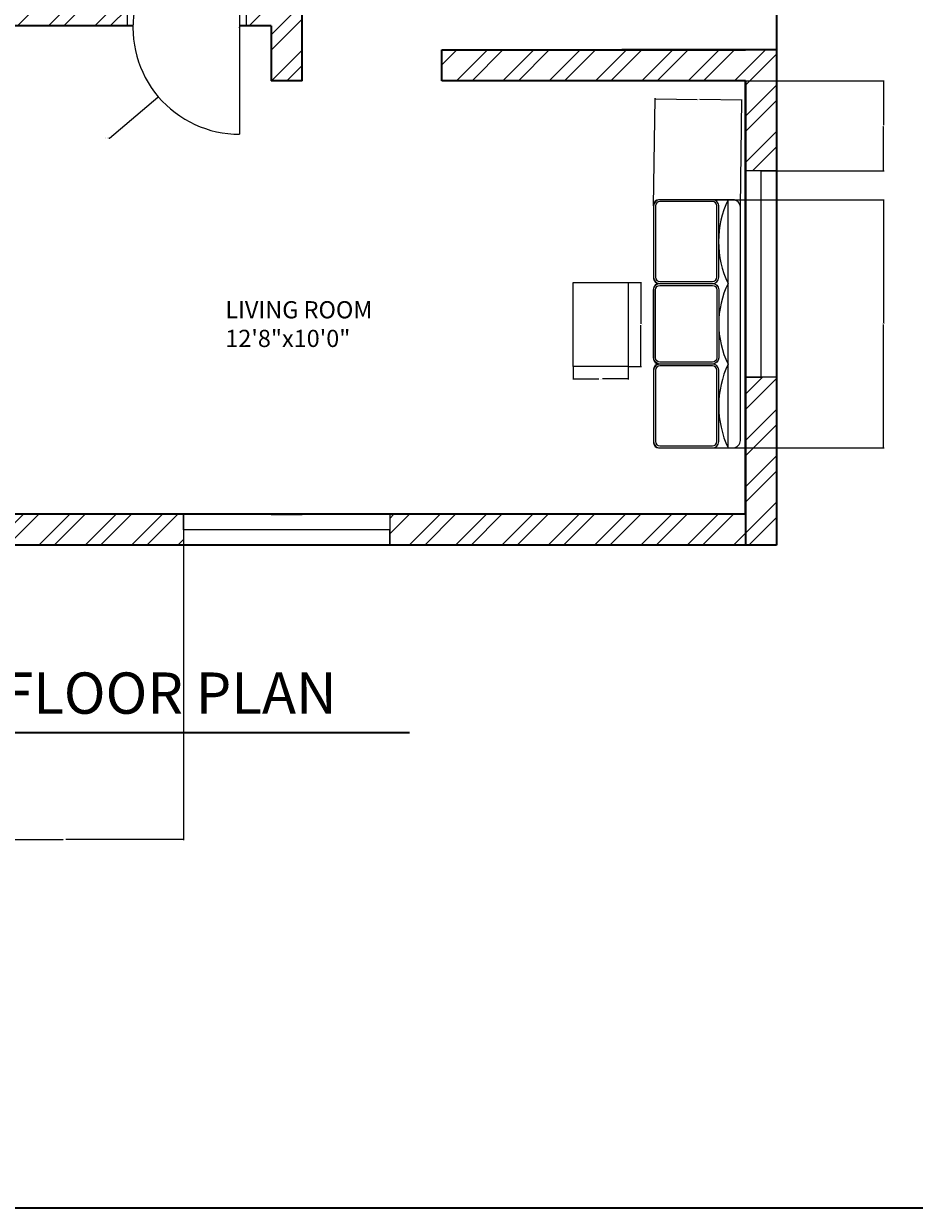
# Model space of a CAD drawing. Units: inches. Extents: x 1955 to 3324, y 980 to 3129.
# Tile 2 of 11: x 2296 to 2555, y 1704 to 2048. Entities that reach past the tile are written whole.
import ezdxf

# ---------------------------------------------------------------- set-up
doc = ezdxf.new("R2010")
doc.units = ezdxf.units.IN
for name, color, linetype, lineweight in [('A-ANNO-DIMS', 2, 'Continuous', 18), ('A-ANNO-TITL', 7, 'Continuous', 35), ('A-ANNO-TTLB', 7, 'Continuous', 35), ('A-AREA-IDEN', 7, 'Continuous', 18), ('A-DOOR', 3, 'Continuous', 18), ('A-FURN', 8, 'Continuous', 18), ('A-GLAZ', 4, 'Continuous', 18), ('A-WALL', 7, 'Continuous', 35), ('A-WALL-PATT', 252, 'Continuous', 13)]:
    doc.layers.add(name, color=color, linetype=linetype, lineweight=lineweight)
doc.styles.get("Standard").update_dxf_attribs({"font": 'arial.ttf'})
doc.dimstyles.get("Standard").update_dxf_attribs({"dimtxt": 0.18, "dimasz": 0.18, "dimexe": 0.18, "dimexo": 0.0625, "dimgap": 0.09, "dimtad": 0, "dimtih": 1, "dimtoh": 1, "dimdec": 4, "dimzin": 0, "dimdsep": 46, "dimtxsty": 'Standard', "dimcen": 0.09, "dimadec": 0, "dimazin": 0, "dimtfac": 1, "dimtdec": 4, "dimtofl": 0, "dimtmove": 0, "dimatfit": 3, "dimfxl": 1, "dimtolj": 1, "dimtzin": 0, "dimarcsym": 0})

# ---------------------------------------------------------------- blocks, each defined once
blk = doc.blocks.new('COFFEE-TABLE-RECT')
blk.add_lwpolyline([(0, 24.35), (16.02, 24.35), (16.02, 0), (0, 0)], close=True)
blk = doc.blocks.new('DOOR-UNIT-S')
for p, q in [((0, 31.5), (0, 40.5)), ((0, 40.5), (0, 36)), ((34.6, 31.5), (34.6, 40.5)), ((34.6, 40.5), (34.6, 36)), ((0, 36), (2, 36)), ((34.6, 36), (32.6, 36)), ((32.6, 36), (32.6, 0))]:
    blk.add_line(p, q)
blk.add_arc((32.6, 31.01), 31.01, 170.7301, 270)
blk = doc.blocks.new('WIN-PLAN-60-A')
for p, q in [((0, 60), (9, 60)), ((9, 60), (4.5, 60)), ((4.5, 60), (4.5, 0)), ((4.5, 0), (0, 0)), ((0, 0), (9, 0))]:
    blk.add_line(p, q)
blk = doc.blocks.new('*D57')
at = {"layer": 'A-ANNO-DIMS', "color": 0, "lineweight": -2, "transparency": 16777216}
for p, q in [((2472.15, 1972.84), (2475.92, 1972.84)), ((2475.74, 1972.66), (2475.74, 1960.85)), ((2475.74, 1948.67), (2475.74, 1960.49)), ((2472.15, 1948.49), (2475.92, 1948.49))]:
    blk.add_line(p, q, dxfattribs=at)
at = {"layer": 'A-ANNO-DIMS', "color": 0, "transparency": 16777216}
for points in [[(2475.71, 1972.66), (2475.77, 1972.66), (2475.74, 1972.84)], [(2475.71, 1948.67), (2475.77, 1948.67), (2475.74, 1948.49)]]:
    blk.add_solid(points, dxfattribs=at)
at = {"layer": 'Defpoints', "color": 0, "transparency": 16777216}
for p in [(2472.09, 1972.84), (2475.74, 1972.84), (2472.09, 1948.49)]:
    blk.add_point(p, dxfattribs=at)
at = {"layer": 'A-ANNO-DIMS', "color": 0, "transparency": 16777216, "insert": (2475.74, 1960.67), "char_height": 0.18, "attachment_point": 5}
blk.add_mtext('\\A1;TABLE 24 TYP.', dxfattribs=at)
blk = doc.blocks.new('*D58')
at = {"layer": 'A-ANNO-DIMS', "color": 0, "lineweight": -2, "transparency": 16777216}
for p, q in [((2456.07, 1948.43), (2456.07, 1944.66)), ((2472.09, 1948.43), (2472.09, 1944.66)), ((2456.25, 1944.84), (2463.56, 1944.84)), ((2471.91, 1944.84), (2464.6, 1944.84))]:
    blk.add_line(p, q, dxfattribs=at)
at = {"layer": 'A-ANNO-DIMS', "color": 0, "transparency": 16777216}
for points in [[(2456.25, 1944.87), (2456.25, 1944.81), (2456.07, 1944.84)], [(2471.91, 1944.87), (2471.91, 1944.81), (2472.09, 1944.84)]]:
    blk.add_solid(points, dxfattribs=at)
at = {"layer": 'Defpoints', "color": 0, "transparency": 16777216}
for p in [(2456.07, 1948.49), (2472.09, 1948.49), (2472.09, 1944.84)]:
    blk.add_point(p, dxfattribs=at)
at = {"layer": 'A-ANNO-DIMS', "color": 0, "transparency": 16777216, "insert": (2464.08, 1944.84), "char_height": 0.18, "attachment_point": 5}
blk.add_mtext('\\A1;16 TYP.', dxfattribs=at)
blk = doc.blocks.new('*D105')
at = {"layer": 'A-ANNO-DIMS', "color": 0, "lineweight": -2, "transparency": 16777216}
for p, q in [((2506.27, 2031.5), (2546.54, 2031.5)), ((2546.36, 2031.32), (2546.36, 2018.62)), ((2546.36, 2005.54), (2546.36, 2018.25)), ((2515.27, 2005.36), (2546.54, 2005.36))]:
    blk.add_line(p, q, dxfattribs=at)
at = {"layer": 'A-ANNO-DIMS', "color": 0, "transparency": 16777216}
for points in [[(2546.33, 2031.32), (2546.39, 2031.32), (2546.36, 2031.5)], [(2546.33, 2005.54), (2546.39, 2005.54), (2546.36, 2005.36)]]:
    blk.add_solid(points, dxfattribs=at)
at = {"layer": 'Defpoints', "color": 0, "transparency": 16777216}
for p in [(2506.21, 2031.5), (2546.36, 2031.5), (2515.21, 2005.36)]:
    blk.add_point(p, dxfattribs=at)
at = {"layer": 'A-ANNO-DIMS', "color": 0, "transparency": 16777216, "insert": (2546.36, 2018.43), "char_height": 0.18, "attachment_point": 5}
blk.add_mtext('\\A1;26.14', dxfattribs=at)
blk = doc.blocks.new('*D109')
at = {"layer": 'A-ANNO-DIMS', "color": 0, "lineweight": -2, "transparency": 16777216}
for p, q in [((2273.49, 1896.44), (2273.49, 1810.7)), ((2342.7, 1896.44), (2342.7, 1810.7)), ((2273.67, 1810.88), (2307.72, 1810.88)), ((2342.52, 1810.88), (2308.47, 1810.88))]:
    blk.add_line(p, q, dxfattribs=at)
at = {"layer": 'A-ANNO-DIMS', "color": 0, "transparency": 16777216}
for points in [[(2273.67, 1810.91), (2273.67, 1810.85), (2273.49, 1810.88)], [(2342.52, 1810.91), (2342.52, 1810.85), (2342.7, 1810.88)]]:
    blk.add_solid(points, dxfattribs=at)
at = {"layer": 'Defpoints', "color": 0, "transparency": 16777216}
for p in [(2273.49, 1896.5), (2342.7, 1896.5), (2342.7, 1810.88)]:
    blk.add_point(p, dxfattribs=at)
at = {"layer": 'A-ANNO-DIMS', "color": 0, "transparency": 16777216, "insert": (2308.09, 1810.88), "char_height": 0.18, "attachment_point": 5}
blk.add_mtext('\\A1;69.21', dxfattribs=at)
blk = doc.blocks.new('*D110')
at = {"layer": 'A-ANNO-DIMS', "color": 0, "lineweight": -2, "transparency": 16777216}
for p, q in [((2479.46, 1995.2), (2479.91, 2026.47)), ((2480.09, 2026.29), (2492.14, 2026.11)), ((2504.98, 2025.93), (2492.93, 2026.1)), ((2504.71, 1994.84), (2505.16, 2026.11))]:
    blk.add_line(p, q, dxfattribs=at)
at = {"layer": 'A-ANNO-DIMS', "color": 0, "transparency": 16777216}
for points in [[(2480.09, 2026.32), (2480.09, 2026.26), (2479.91, 2026.29)], [(2504.98, 2025.96), (2504.97, 2025.9), (2505.16, 2025.93)]]:
    blk.add_solid(points, dxfattribs=at)
at = {"layer": 'Defpoints', "color": 0, "transparency": 16777216}
for p in [(2505.16, 2025.93), (2479.46, 1995.14), (2504.71, 1994.78)]:
    blk.add_point(p, dxfattribs=at)
at = {"layer": 'A-ANNO-DIMS', "color": 0, "transparency": 16777216, "insert": (2492.53, 2026.11), "char_height": 0.18, "attachment_point": 5}
blk.add_mtext('\\A1;25.25', dxfattribs=at)
blk = doc.blocks.new('*D111')
at = {"layer": 'A-ANNO-DIMS', "color": 0, "lineweight": -2, "transparency": 16777216}
for p, q in [((2496.66, 1996.94), (2546.54, 1996.94)), ((2546.36, 1996.76), (2546.36, 1961.06)), ((2546.36, 1924.99), (2546.36, 1960.7)), ((2496.66, 1924.81), (2546.54, 1924.81))]:
    blk.add_line(p, q, dxfattribs=at)
at = {"layer": 'A-ANNO-DIMS', "color": 0, "transparency": 16777216}
for points in [[(2546.33, 1996.76), (2546.39, 1996.76), (2546.36, 1996.94)], [(2546.33, 1924.99), (2546.39, 1924.99), (2546.36, 1924.81)]]:
    blk.add_solid(points, dxfattribs=at)
at = {"layer": 'Defpoints', "color": 0, "transparency": 16777216}
for p in [(2496.6, 1996.94), (2546.36, 1996.94), (2496.6, 1924.81)]:
    blk.add_point(p, dxfattribs=at)
at = {"layer": 'A-ANNO-DIMS', "color": 0, "transparency": 16777216, "insert": (2546.36, 1960.88), "char_height": 0.18, "attachment_point": 5}
blk.add_mtext('\\A1;72.13', dxfattribs=at)
blk = doc.blocks.new('*D140')
at = {"layer": 'A-ANNO-DIMS', "color": 0, "lineweight": -2, "transparency": 16777216}
for p, q in [((2358.92, 2047), (2359.1, 2047)), ((2359.01, 2046.91), (2359.01, 2047.09)), ((2321.21, 2014.87), (2335.25, 2026.8)), ((2321.03, 2014.87), (2321.21, 2014.87))]:
    blk.add_line(p, q, dxfattribs=at)
at = {"layer": 'A-ANNO-DIMS', "color": 0, "transparency": 16777216}
blk.add_solid([(2335.23, 2026.82), (2335.27, 2026.78), (2335.39, 2026.92)], dxfattribs=at)
at = {"layer": 'Defpoints', "color": 0, "transparency": 16777216}
for p in [(2359.01, 2047), (2335.39, 2026.92)]:
    blk.add_point(p, dxfattribs=at)
at = {"layer": 'A-ANNO-DIMS', "color": 0, "transparency": 16777216, "insert": (2320.48, 2014.87), "char_height": 0.18, "attachment_point": 5}
blk.add_mtext('\\A1;R31.005', dxfattribs=at)

msp = doc.modelspace()

# ---------------------------------------------------------------- hatches: boundary and pattern name
at = {"layer": 'A-WALL-PATT'}
h = msp.add_hatch(dxfattribs=at)
h.set_pattern_fill('ANSI32', color=256)
h.paths.add_polyline_path([(2361.4775, 2456.5037), (2270.2755, 2456.5037), (2270.2755, 2447.5037), (2285.7102, 2447.5037), (2285.7102, 2363.5037), (2281.1795, 2363.5037), (2281.1795, 2359.0037), (2290.2102, 2359.0037), (2290.2102, 2447.5037), (2361.4775, 2447.5037), (2361.4775, 2452.0037)])
h.paths.add_polyline_path([(2246.2755, 2456.5037), (2197.6809, 2456.5037), (2197.6809, 2447.5037), (2233.2102, 2447.5037), (2233.2102, 2355.6044), (2237.7102, 2355.6044), (2237.7102, 2447.5037), (2246.2755, 2447.5037)], flags=17)
h.paths.add_polyline_path([(2137.6809, 2456.5037), (2110.2102, 2456.5037), (2110.2102, 2312.5037), (2152.2102, 2312.5037), (2281.2102, 2312.5037), (2281.2102, 2107.6185), (2290.2102, 2107.6185), (2290.2102, 2267.9289), (2329.216, 2267.9289), (2329.216, 2272.4289), (2329.216, 2276.9289), (2290.2102, 2276.9289), (2290.2102, 2321.5037), (2281.2102, 2321.5037), (2119.2102, 2321.5037), (2119.2102, 2447.5037), (2137.6809, 2447.5037)])
h.paths.add_polyline_path([(2515.2102, 2456.5037), (2421.4775, 2456.5037), (2421.4775, 2447.5037), (2506.2102, 2447.5037), (2506.2102, 2415.6626), (2515.2102, 2415.6626)])
h.paths.add_polyline_path([(2515.2102, 2355.6626), (2506.2102, 2355.6626), (2506.2102, 2321.5037), (2424.9282, 2321.5037), (2424.9282, 2312.5037), (2461.2102, 2312.5037), (2470.2102, 2312.5037), (2515.2102, 2312.5037)])
h.paths.add_polyline_path([(2515.2102, 2232.5037), (2470.2102, 2232.5037), (2470.2102, 2237.3759), (2465.7102, 2237.3759), (2461.2102, 2237.3759), (2461.2102, 2232.5037), (2377.2219, 2232.5037), (2377.2219, 2321.5037), (2368.2219, 2321.5037), (2368.2219, 2276.9289), (2359.3802, 2276.9289), (2359.3802, 2272.4289), (2359.3802, 2267.9289), (2368.2219, 2267.9289), (2368.2219, 2223.5037), (2377.2219, 2223.5037), (2461.2102, 2223.5037), (2506.2102, 2223.5037), (2506.2102, 2129.5037), (2461.2102, 2129.5037), (2387.2102, 2129.5037), (2368.2219, 2129.5037), (2368.2219, 2056.4936), (2361.0095, 2056.4936), (2361.0095, 2051.9936), (2361.0095, 2047.4936), (2368.2219, 2047.4936), (2368.2219, 2031.5037), (2377.2219, 2031.5037), (2377.2219, 2120.5037), (2461.2102, 2120.5037), (2461.2102, 2112.7921), (2470.2102, 2112.7921), (2470.2102, 2120.5037), (2515.2102, 2120.5037), (2515.2102, 2129.5037)])
h.paths.add_polyline_path([(2470.2102, 2277.1758), (2461.2102, 2277.1758), (2461.2102, 2272.5037), (2461.2102, 2270.2549), (2470.2102, 2270.2549), (2470.2102, 2272.5037)], flags=17)
h.paths.add_polyline_path([(2515.2102, 2040.5037), (2470.2102, 2040.5037), (2417.8264, 2040.5037), (2417.8264, 2031.5037), (2506.2102, 2031.5037), (2506.2102, 2005.3639), (2515.2102, 2005.3639)])
h.paths.add_polyline_path([(2506.2102, 1905.5037), (2402.6963, 1905.5037), (2402.6963, 1896.5037), (2506.2102, 1896.5037)])
h.paths.add_polyline_path([(2515.2102, 1945.3639), (2506.2102, 1945.3639), (2506.2102, 1905.5037), (2506.2102, 1896.5037), (2515.2102, 1896.5037)])
h.paths.add_polyline_path([(2342.6963, 1901.0037), (2342.6963, 1905.5037), (2273.4892, 1905.5037), (2273.4892, 1896.5037), (2342.6963, 1896.5037)])
h.paths.add_polyline_path([(2290.2102, 1994.0037), (2283.612, 1994.0037), (2283.612, 1991.7537), (2283.612, 1989.5037), (2285.7102, 1989.5037), (2285.7102, 1905.5037), (2290.2102, 1905.5037)])
h.paths.add_polyline_path([(2249.4892, 1905.5037), (2237.7102, 1905.5037), (2206.3617, 1905.5037), (2206.3617, 1896.5037), (2249.4892, 1896.5037), (2249.4892, 1901.0037)])
h.paths.add_polyline_path([(2237.7102, 1989.5037), (2261.7102, 1989.5037), (2261.7102, 1994.0037), (2237.7102, 1994.0037), (2237.7102, 1999.266), (2235.4602, 1999.266), (2233.2102, 1999.266), (2233.2102, 1994.0037), (2233.2102, 1905.5037), (2237.7102, 1905.5037)])
h.paths.add_polyline_path([(2119.2102, 1947.5144), (2110.2102, 1947.5144), (2110.2102, 1896.5037), (2119.2102, 1896.5037), (2146.3617, 1896.5037), (2146.3617, 1901.0037), (2146.3617, 1905.5037), (2119.2102, 1905.5037)])
h.paths.add_polyline_path([(2119.2102, 2068.6379), (2110.2102, 2068.6379), (2110.2102, 2007.5144), (2119.2102, 2007.5144), (2119.2102, 2031.5037), (2233.2102, 2031.5037), (2233.2102, 2027.9287), (2235.4602, 2027.9287), (2237.7102, 2027.9287), (2237.7102, 2031.5037), (2281.2102, 2031.5037), (2290.2102, 2031.5037), (2290.2102, 2047.4936), (2326.409, 2047.4936), (2326.409, 2056.4936), (2290.2102, 2056.4936), (2290.2102, 2071.2722), (2285.7102, 2071.2722), (2281.2102, 2071.2722), (2281.2102, 2040.5037), (2227.2102, 2040.5037), (2227.2102, 2111.2571), (2222.7102, 2111.2571), (2218.2102, 2111.2571), (2218.2102, 2040.5037), (2119.2102, 2040.5037)])
h.paths.add_polyline_path([(2236.9166, 2214.5037), (2161.2102, 2214.5037), (2161.2102, 2221.6488), (2152.2102, 2221.6488), (2152.2102, 2214.5037), (2110.2102, 2214.5037), (2110.2102, 2205.5037), (2131.2394, 2205.5037), (2131.2394, 2198.3478), (2140.2394, 2198.3478), (2140.2394, 2205.5037), (2224.2394, 2205.5037), (2224.2394, 2200.2317), (2228.7394, 2200.2317), (2233.2394, 2200.2317), (2233.2394, 2205.5037), (2236.9166, 2205.5037)], flags=17)
h.paths.add_polyline_path([(2236.9166, 2157.5037), (2233.2394, 2157.5037), (2233.2394, 2178.9172), (2228.7394, 2178.9172), (2224.2394, 2178.9172), (2224.2394, 2157.5037), (2140.2394, 2157.5037), (2140.2394, 2174.3478), (2131.2394, 2174.3478), (2131.2394, 2157.5037), (2110.2102, 2157.5037), (2110.2102, 2128.6379), (2119.2102, 2128.6379), (2119.2102, 2148.5037), (2218.2102, 2148.5037), (2218.2102, 2141.7262), (2222.7102, 2141.7262), (2227.2102, 2141.7262), (2227.2102, 2148.5037), (2236.9166, 2148.5037)], flags=0)
h.paths.add_polyline_path([(3084.7449, 2537.3808), (3212.7954, 2537.3808), (3212.7954, 2555.9271), (3084.7449, 2555.9271)], flags=9)
h.paths.add_polyline_path([(3068.7485, 2853.43), (3169.977, 2853.43), (3169.977, 2871.9764), (3068.7485, 2871.9764)], flags=9)
h.paths.add_polyline_path([(3074.1798, 2918.0252), (3126.4732, 2918.0252), (3126.4732, 2936.5716), (3074.1798, 2936.5716)], flags=9)
h.paths.add_polyline_path([(3073.0928, 2947.3127), (3199.0499, 2947.3127), (3199.0499, 2965.8591), (3073.0928, 2965.8591)], flags=9)
h.paths.add_polyline_path([(2733.8393, 2484.8678), (2879.7915, 2484.8678), (2879.7915, 2521.9606), (2733.8393, 2521.9606)], flags=9)
h.paths.add_polyline_path([(2204.9881, 2482.4168), (2355.1272, 2482.4168), (2355.1272, 2519.5095), (2204.9881, 2519.5095)], flags=9)
h.paths.add_polyline_path([(3062.1429, 2387.2466), (3079.3735, 2387.2466), (3079.3735, 2411.9751), (3062.1429, 2411.9751)], flags=9)
h.paths.add_polyline_path([(2190.1574, 2158.8439), (2219.315, 2158.8439), (2219.315, 2177.5013), (2190.1574, 2177.5013)], flags=25)
h.paths.add_polyline_path([(2213.6766, 1840.7276), (2405.0382, 1840.7276), (2405.0382, 1865.4561), (2213.6766, 1865.4561)], flags=9)
h.paths.add_polyline_path([(2180.5398, 2233.911), (2213.9471, 2233.911), (2213.9471, 2252.5683), (2180.5398, 2252.5683)], flags=25)
h.paths.add_polyline_path([(2134.4484, 2238.3973), (2134.4484, 2274.2807), (2115.791, 2274.2807), (2115.791, 2238.3973)], flags=25)
h.paths.add_polyline_path([(2135.1593, 2122.9991), (2173.7507, 2122.9991), (2173.7507, 2141.6565), (2135.1593, 2141.6565)], flags=25)
h.paths.add_polyline_path([(2129.8822, 2002.1912), (2168.4736, 2002.1912), (2168.4736, 2020.8486), (2129.8822, 2020.8486)], flags=9)
h.paths.add_polyline_path([(2239.6647, 1953.4107), (2268.8973, 1953.4107), (2268.8973, 1972.068), (2239.6647, 1972.068)], flags=9)
h.paths.add_polyline_path([(2352.8562, 1951.2904), (2402.1775, 1951.2904), (2402.1775, 1969.9477), (2352.8562, 1969.9477)], flags=9)
h.paths.add_polyline_path([(2500.1358, 2055.32), (2500.1358, 2091.2034), (2481.4784, 2091.2034), (2481.4784, 2055.32)], flags=25)
h.paths.add_polyline_path([(2391.2702, 2058.6821), (2424.4285, 2058.6821), (2424.4285, 2077.3394), (2391.2702, 2077.3394)], flags=25)
h.paths.add_polyline_path([(2507.7996, 2257.2758), (2507.7996, 2293.1592), (2489.1422, 2293.1592), (2489.1422, 2257.2758)], flags=25)
h.paths.add_polyline_path([(2386.8349, 2273.8734), (2419.9931, 2273.8734), (2419.9931, 2292.5307), (2386.8349, 2292.5307)], flags=25)
h.paths.add_polyline_path([(2335.374, 2373.3267), (2384.6953, 2373.3267), (2384.6953, 2391.984), (2335.374, 2391.984)], flags=9)
h.paths.add_polyline_path([(2243.8205, 2380.6539), (2273.0531, 2380.6539), (2273.0531, 2399.3113), (2243.8205, 2399.3113)], flags=25)
h.paths.add_polyline_path([(2126.2627, 2321.6894), (2164.8541, 2321.6894), (2164.8541, 2340.3467), (2126.2627, 2340.3467)], flags=25)

# ---------------------------------------------------------------- linework, layer by layer
at = {"layer": 'A-ANNO-TITL'}
msp.add_line((2209.2481, 1842.0268), (2408.4415, 1842.0268), dxfattribs=at)
at = {"layer": 'A-ANNO-TTLB'}
msp.add_lwpolyline([(1954.5391, 3128.9103), (3323.9705, 3128.9103), (3323.9705, 1703.6826), (1954.5391, 1703.6826)], close=True, dxfattribs=at)
at = {"layer": 'A-FURN'}
for points in [[(2481.267, 1972.5997), (2496.5952, 1972.5997, 0.41421356), (2498.3986, 1974.403), (2498.3986, 1995.1412, 0.41421356), (2496.5952, 1996.9445), (2481.267, 1996.9445, 0.41421356), (2479.4637, 1995.1412), (2479.4637, 1974.403, 0.41421356)], [(2481.267, 1973.1407), (2496.5952, 1973.1407, 0.41421356), (2497.8576, 1974.403), (2497.8576, 1995.1412, 0.41421356), (2496.5952, 1996.4035), (2481.267, 1996.4035, 0.41421356), (2480.0047, 1995.1412), (2480.0047, 1974.403, 0.41421356)], [(2481.267, 1972.5997), (2496.5952, 1972.5997, -0.41421356), (2498.3986, 1970.7963), (2498.3986, 1950.9598, -0.41421356), (2496.5952, 1949.1565), (2481.267, 1949.1565, -0.41421356), (2479.4637, 1950.9598), (2479.4637, 1970.7963, -0.41421356)], [(2481.267, 1972.0587), (2496.5952, 1972.0587, -0.41421356), (2497.8576, 1970.7963), (2497.8576, 1950.9598, -0.41421356), (2496.5952, 1949.6975), (2481.267, 1949.6975, -0.41421356), (2480.0047, 1950.9598), (2480.0047, 1970.7963, -0.41421356)], [(2481.267, 1924.8117), (2496.5952, 1924.8117, 0.41421356), (2498.3986, 1926.615), (2498.3986, 1947.3532, 0.41421356), (2496.5952, 1949.1565), (2481.267, 1949.1565, 0.41421356), (2479.4637, 1947.3532), (2479.4637, 1926.615, 0.41421356)], [(2481.267, 1925.3527), (2496.5952, 1925.3527, 0.41421356), (2497.8576, 1926.615), (2497.8576, 1947.3532, 0.41421356), (2496.5952, 1948.6155), (2481.267, 1948.6155, 0.41421356), (2480.0047, 1947.3532), (2480.0047, 1926.615, 0.41421356)]]:
    msp.add_lwpolyline(points, format="xyb", close=True, dxfattribs=at)
at = {"layer": 'A-FURN', "ltscale": 0.03}
msp.add_lwpolyline([(2479.4637, 1947.6961), (2479.4637, 1926.2543, 0.41421356), (2480.9063, 1924.8117), (2502.5462, 1924.8117, 0.41421356), (2504.7102, 1926.9756), (2504.7102, 1994.7805, 0.41421356), (2502.5462, 1996.9445), (2480.9063, 1996.9445, 0.41421356), (2479.4637, 1995.5018), (2479.4637, 1974.0601, 0.41421356), (2480.9063, 1972.6174, -1), (2480.9063, 1972.5819, 0.41421356), (2479.4637, 1971.1393), (2479.4637, 1950.6169, 0.41421356), (2480.9063, 1949.1742, -1), (2480.9063, 1949.1388, 0.41421356)], format="xyb", close=True, dxfattribs=at)
at = {"layer": 'A-FURN'}
msp.add_lwpolyline([(2501.1035, 1924.8117), (2501.1035, 1996.9445)], dxfattribs=at)
for centre, radius, start, end in [((2526.8009, 1984.7721), 28.4345, 154.653824, 205.346176), ((2524.9975, 1960.8781), 26.6143, 153.868999, 206.131001), ((2527.1014, 1936.9841), 28.7064, 154.910626, 205.089374)]:
    msp.add_arc(centre, radius, start, end, dxfattribs=at)
at = {"layer": 'A-WALL'}
for p, q in [((2515.2102, 2456.5037), (2515.2102, 1896.5037)), ((2377.2219, 2031.5037), (2377.2219, 2120.5037)), ((2328.008, 2047.4936), (2290.2102, 2047.4936)), ((2368.2219, 2047.4936), (2359.0095, 2047.4936)), ((2368.2219, 2047.4936), (2368.2219, 2031.5037)), ((2417.8264, 2031.5037), (2417.8264, 2040.5037)), ((2417.8264, 2040.5037), (2506.2102, 2040.5037)), ((2515.2102, 2040.5037), (2470.2102, 2040.5037)), ((2377.2219, 2031.5037), (2368.2219, 2031.5037)), ((2506.2102, 2031.5037), (2417.8264, 2031.5037)), ((2506.2102, 1905.5037), (2506.2102, 2031.5037)), ((2506.2102, 2031.5037), (2506.2102, 1896.5037)), ((2506.2102, 1905.5037), (2119.2102, 1905.5037)), ((2368.2219, 1905.5037), (2377.2219, 1905.5037)), ((2515.2102, 1896.5037), (2110.2102, 1896.5037))]:
    msp.add_line(p, q, dxfattribs=at)

# ---------------------------------------------------------------- block references
at = {"layer": 'A-DOOR'}
msp.add_blockref('DOOR-UNIT-S', (2326.409, 2015.994), dxfattribs=at)
at = {"layer": 'A-FURN'}
msp.add_blockref('COFFEE-TABLE-RECT', (2456.067, 1948.492), dxfattribs=at)
at = {"layer": 'A-GLAZ'}
for p, rotation in [((2515.2105, 2005.3635), 180), ((2342.6968, 1905.5039), 270.0000000000005)]:
    msp.add_blockref('WIN-PLAN-60-A', p, dxfattribs=dict(at, rotation=rotation))

# ---------------------------------------------------------------- texts
at = {"layer": 'A-ANNO-TITL', "insert": (2217.5689, 1859.4929), "char_height": 12, "attachment_point": 1}
msp.add_mtext_dynamic_manual_height_columns('GROUND FLOOR PLAN', width=433.353325, gutter_width=12.5, heights=[0], dxfattribs=at)
at = {"layer": 'A-AREA-IDEN', "insert": (2354.8668, 1967.4631), "char_height": 5, "attachment_point": 1}
msp.add_mtext_dynamic_manual_height_columns('LIVING ROOM\\P12\'8"x10\'0"', width=115.225682, gutter_width=12.5, heights=[0], dxfattribs=at)

# ---------------------------------------------------------------- dimensions: what is measured, and where the dimension line sits
at = {"layer": 'A-ANNO-DIMS'}
dim = msp.add_radius_dim(center=(2359.0095, 2046.9991), mpoint=(2335.3854, 2026.9183), dimstyle='Standard', override={"dimdec": 3, "dimlfac": 1, "dimrnd": 0, "dimzin": 0, "dimdsep": 46, "dimlunit": 2}, dxfattribs=at)
dim.commit()
dim.dimension.update_dxf_attribs({"geometry": '*D140', "text_midpoint": (2320.4804, 2014.8698), "dimtype": 164})
for base, p1, p2, angle, picture, middle in [((2546.3602, 2031.5037), (2515.2102, 2005.3639), (2506.2102, 2031.5037), 90, '*D105', (2546.3602, 2018.4338)), ((2505.1551, 2025.9273), (2479.4637, 1995.1412), (2504.7102, 1994.7805), 359.181545, '*D110', (2492.5319, 2026.1077)), ((2546.3602, 1996.9445), (2496.5952, 1924.8117), (2496.5952, 1996.9445), 90, '*D111', (2546.3602, 1960.8781))]:
    dim = msp.add_linear_dim(base=base, p1=p1, p2=p2, angle=angle, dimstyle='Standard', override={"dimdec": 2, "dimlfac": 1, "dimrnd": 0, "dimzin": 0, "dimdsep": 46, "dimlunit": 2}, dxfattribs=at)
    dim.commit()
    dim.dimension.update_dxf_attribs({"geometry": picture, "text_midpoint": middle})
dim = msp.add_linear_dim(base=(2475.742, 1972.8417), p1=(2472.0895, 1948.4918), p2=(2472.0895, 1972.8417), angle=90, text='TABLE <> TYP.', dimstyle='Standard', override={"dimdec": 0, "dimlfac": 1, "dimrnd": 0, "dimzin": 0, "dimdsep": 46, "dimlunit": 2}, dxfattribs=at)
dim.commit()
dim.dimension.update_dxf_attribs({"geometry": '*D57', "text_midpoint": (2475.742, 1960.6667)})
dim = msp.add_linear_dim(base=(2472.0895, 1944.8393), p1=(2456.0666, 1948.4918), p2=(2472.0895, 1948.4918), text='<> TYP.', dimstyle='Standard', override={"dimdec": 0, "dimlfac": 1, "dimrnd": 0, "dimzin": 0, "dimdsep": 46, "dimlunit": 2}, dxfattribs=at)
dim.commit()
dim.dimension.update_dxf_attribs({"geometry": '*D58', "text_midpoint": (2464.0781, 1944.8393)})
dim = msp.add_linear_dim(base=(2342.6963, 1810.8768), p1=(2273.4892, 1896.5037), p2=(2342.6963, 1896.5037), dimstyle='Standard', override={"dimdec": 2, "dimlfac": 1, "dimrnd": 0, "dimzin": 0, "dimdsep": 46, "dimlunit": 2}, dxfattribs=at)
dim.commit()
dim.dimension.update_dxf_attribs({"geometry": '*D109', "text_midpoint": (2308.0927, 1810.8768)})

doc.saveas('drawing.dxf')
